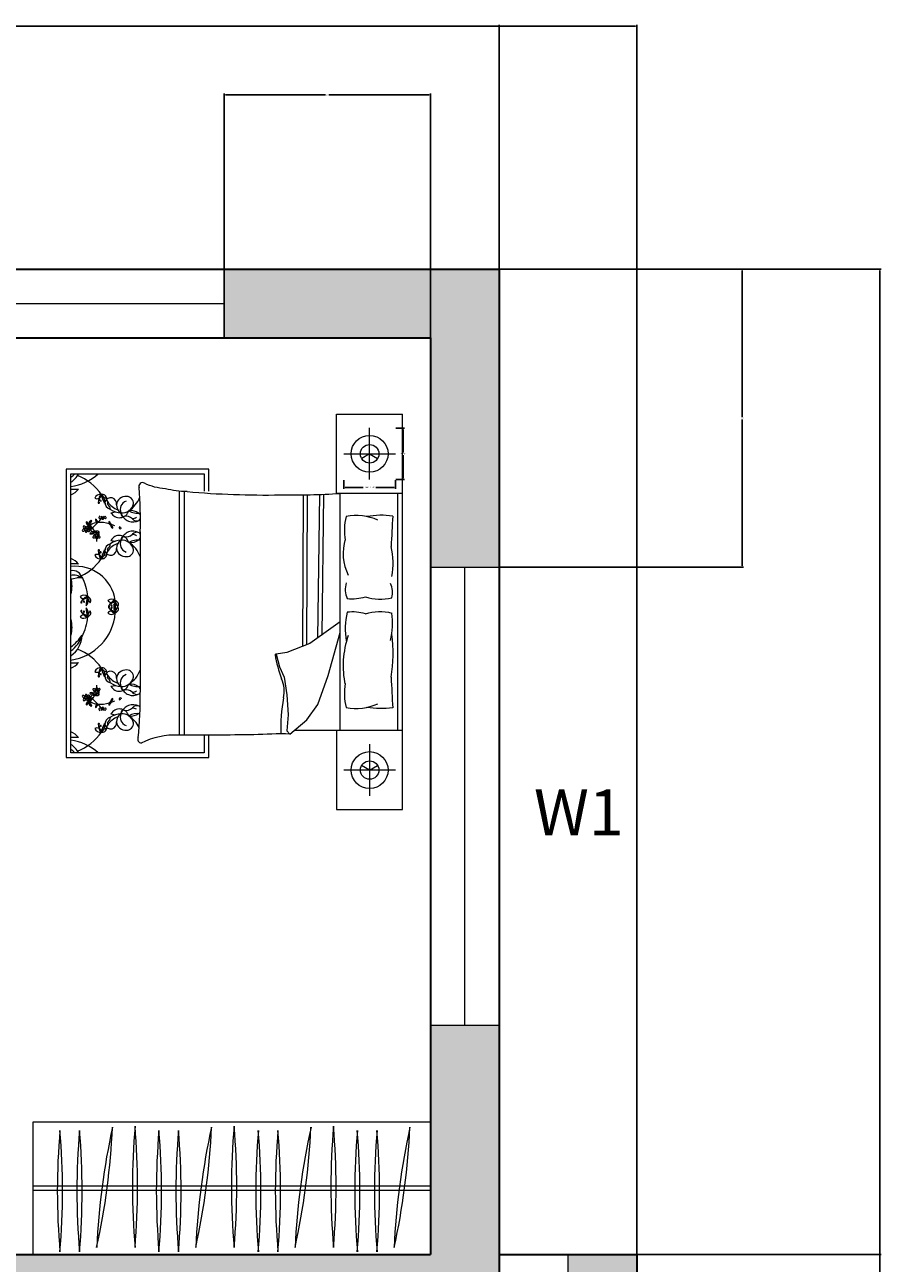
# Model space of a CAD drawing. Units: inches. Extents: x 5 to 421, y -617 to 43.
# Tile 15 of 15: x 308 to 421, y -119 to 43. Entities that reach past the tile are written whole.
import ezdxf

# ---------------------------------------------------------------- set-up
doc = ezdxf.new("R2010")
doc.units = ezdxf.units.IN
doc.header["$MEASUREMENT"] = 0
for name, color, linetype, lineweight in [('A-ANNO-DIMS', 2, 'Continuous', 18), ('A-ANNO-TEXT', 7, 'Continuous', 18), ('A-FLOR-CASE', 8, 'Continuous', 18), ('A-FURN', 8, 'Continuous', 13), ('A-GLAZ', 4, 'Continuous', 18), ('A-WALL', 7, 'Continuous', 35)]:
    doc.layers.add(name, color=color, linetype=linetype, lineweight=lineweight)
doc.layers.add('A-WALL-PATT', color=251, linetype='Continuous', lineweight=13, true_color=0x636466)
doc.styles.get("Standard").update_dxf_attribs({"font": 'arial.ttf'})
doc.dimstyles.get("Standard").update_dxf_attribs({"dimtxt": 0.18, "dimasz": 0.18, "dimexe": 0.18, "dimexo": 0.0625, "dimgap": 0.09, "dimtad": 0, "dimtih": 1, "dimtoh": 1, "dimdec": 0, "dimzin": 0, "dimdsep": 46, "dimlunit": 3, "dimtxsty": 'Standard', "dimcen": 0.09, "dimadec": 0, "dimazin": 0, "dimtfac": 1, "dimtdec": 0, "dimtofl": 0, "dimtmove": 0, "dimatfit": 3, "dimfxl": 1, "dimtolj": 1, "dimtzin": 0, "dimarcsym": 0})

# ---------------------------------------------------------------- blocks, each defined once
blk = doc.blocks.new('WINDOW-W1-60')
for p, q in [((0, 9), (60, 9)), ((0, 0), (0, 9)), ((60, 9), (60, 0)), ((0, 4.5), (60, 4.5)), ((60, 0), (0, 0))]:
    blk.add_line(p, q)
blk = doc.blocks.new('WARDROBE-52')
for p, q in [((52, 17.33), (0, 17.33)), ((0, 17.33), (0, 0)), ((52, 17.33), (52, 0)), ((52, 8.96), (0, 8.96)), ((52, 8.38), (0, 8.38)), ((52, 0), (0, 0))]:
    blk.add_line(p, q)
for centre, start, end in [((94.39, 8.32), 175.0028, 184.9972), ((-87.33, 8.32), 355.0028, 4.9972), ((96.95, 8.32), 175.0028, 184.9972), ((-84.76, 8.32), 355.0028, 4.9972), ((-80.71, 20.66), 347.508, 357.5023), ((99.46, -3.04), 167.508, 177.5023), ((104.22, 8.88), 175.0028, 184.9972), ((-77.5, 8.88), 355.0028, 4.9972), ((107.34, 8.32), 175.0028, 184.9972), ((-74.38, 8.32), 355.0028, 4.9972), ((109.91, 8.32), 175.0028, 184.9972), ((-71.81, 8.32), 355.0028, 4.9972), ((-67.75, 20.66), 347.508, 357.5023), ((112.41, -3.04), 167.508, 177.5023), ((117.17, 8.88), 175.0028, 184.9972), ((-64.54, 8.88), 355.0028, 4.9972), ((120.35, 8.32), 175.0028, 184.9972), ((-61.37, 8.32), 355.0028, 4.9972), ((122.91, 8.32), 175.0028, 184.9972), ((-58.8, 8.32), 355.0028, 4.9972), ((125.42, -3.04), 167.508, 177.5023), ((-54.75, 20.66), 347.508, 357.5023), ((130.18, 8.88), 175.0028, 184.9972), ((-51.54, 8.88), 355.0028, 4.9972), ((133.3, 8.32), 175.0028, 184.9972), ((-48.42, 8.32), 355.0028, 4.9972), ((135.87, 8.32), 175.0028, 184.9972), ((-45.85, 8.32), 355.0028, 4.9972), ((138.37, -3.04), 167.508, 177.5023), ((-41.79, 20.66), 347.508, 357.5023)]:
    blk.add_arc(centre, 91.2, start, end)
blk = doc.blocks.new('BEDSIDE-LAMP-SINGLE')
for p, q in [((3.38, 0), (3.38, 6.76)), ((0, 3.38), (6.76, 3.38))]:
    blk.add_line(p, q)
for points in [[(3.38, 3.38), (2.34, 2.78)], [(3.38, 3.38), (4.43, 2.78)]]:
    blk.add_lwpolyline(points)
for radius in [2.41, 1.21]:
    blk.add_circle((3.38, 3.38), radius)
blk = doc.blocks.new('*D50')
at = {"layer": 'A-ANNO-DIMS', "color": 0, "lineweight": -2, "transparency": 16777216}
for p, q in [((350.09, -16.74), (350.09, -17.87)), ((350.27, -17.69), (352.64, -17.69)), ((356.67, -17.69), (354.3, -17.69)), ((356.85, -16.74), (356.85, -17.87))]:
    blk.add_line(p, q, dxfattribs=at)
at = {"layer": 'A-ANNO-DIMS', "color": 0, "transparency": 16777216}
for points in [[(350.27, -17.66), (350.27, -17.72), (350.09, -17.69)], [(356.67, -17.66), (356.67, -17.72), (356.85, -17.69)]]:
    blk.add_solid(points, dxfattribs=at)
at = {"layer": 'Defpoints', "color": 0, "transparency": 16777216}
for p in [(350.09, -16.68), (356.85, -16.68), (356.85, -17.69)]:
    blk.add_point(p, dxfattribs=at)
at = {"layer": 'A-ANNO-DIMS', "color": 0, "transparency": 16777216, "insert": (353.47, -17.69), "char_height": 0.18, "attachment_point": 5}
blk.add_mtext('\\A1;LAMP 7 TYP.', dxfattribs=at)
blk = doc.blocks.new('*D51')
at = {"layer": 'A-ANNO-DIMS', "color": 0, "lineweight": -2, "transparency": 16777216}
for p, q in [((356.91, -9.92), (358.04, -9.92)), ((357.86, -10.1), (357.86, -13.12)), ((357.86, -16.5), (357.86, -13.48)), ((356.91, -16.68), (358.04, -16.68))]:
    blk.add_line(p, q, dxfattribs=at)
at = {"layer": 'A-ANNO-DIMS', "color": 0, "transparency": 16777216}
for points in [[(357.83, -10.1), (357.89, -10.1), (357.86, -9.92)], [(357.83, -16.5), (357.89, -16.5), (357.86, -16.68)]]:
    blk.add_solid(points, dxfattribs=at)
at = {"layer": 'Defpoints', "color": 0, "transparency": 16777216}
for p in [(356.85, -9.92), (357.86, -9.92), (356.85, -16.68)]:
    blk.add_point(p, dxfattribs=at)
at = {"layer": 'A-ANNO-DIMS', "color": 0, "transparency": 16777216, "insert": (357.86, -13.3), "char_height": 0.18, "attachment_point": 5}
blk.add_mtext('\\A1;7 TYP.', dxfattribs=at)
blk = doc.blocks.new('*D54')
at = {"layer": 'A-ANNO-DIMS', "color": 0, "lineweight": -2, "transparency": 16777216}
for p, q in [((37.42, 10.94), (37.42, 42.86)), ((37.6, 42.68), (212.65, 42.68)), ((388.24, 42.68), (213.19, 42.68)), ((388.42, -118.06), (388.42, 42.86))]:
    blk.add_line(p, q, dxfattribs=at)
at = {"layer": 'A-ANNO-DIMS', "color": 0, "transparency": 16777216}
for points in [[(37.6, 42.71), (37.6, 42.65), (37.42, 42.68)], [(388.24, 42.71), (388.24, 42.65), (388.42, 42.68)]]:
    blk.add_solid(points, dxfattribs=at)
at = {"layer": 'Defpoints', "color": 0, "transparency": 16777216}
for p in [(37.42, 42.68), (37.42, 10.88), (388.42, -118.12)]:
    blk.add_point(p, dxfattribs=at)
at = {"layer": 'A-ANNO-DIMS', "color": 0, "transparency": 16777216, "insert": (212.92, 42.68), "char_height": 0.18, "attachment_point": 5}
blk.add_mtext('\\A1;351', dxfattribs=at)
blk = doc.blocks.new('*D55')
at = {"layer": 'A-ANNO-DIMS', "color": 0, "lineweight": -2, "transparency": 16777216}
for p, q in [((370.48, 10.88), (420.4, 10.88)), ((420.22, 10.7), (420.22, -286.69)), ((420.22, -584.44), (420.22, -287.05)), ((169.48, -584.62), (420.4, -584.62))]:
    blk.add_line(p, q, dxfattribs=at)
at = {"layer": 'A-ANNO-DIMS', "color": 0, "transparency": 16777216}
for points in [[(420.19, 10.7), (420.25, 10.7), (420.22, 10.88)], [(420.19, -584.44), (420.25, -584.44), (420.22, -584.62)]]:
    blk.add_solid(points, dxfattribs=at)
at = {"layer": 'Defpoints', "color": 0, "transparency": 16777216}
for p in [(370.42, 10.88), (169.42, -584.62), (420.22, -584.62)]:
    blk.add_point(p, dxfattribs=at)
at = {"layer": 'A-ANNO-DIMS', "color": 0, "transparency": 16777216, "insert": (420.22, -286.87), "char_height": 0.18, "attachment_point": 5}
blk.add_mtext('\\A1;595.5', dxfattribs=at)
blk = doc.blocks.new('*D58')
at = {"layer": 'A-ANNO-DIMS', "color": 0, "lineweight": -2, "transparency": 16777216}
for p, q in [((334.42, 1.94), (334.42, 33.86)), ((334.6, 33.68), (347.7, 33.68)), ((361.24, 33.68), (348.14, 33.68)), ((361.42, 1.94), (361.42, 33.86))]:
    blk.add_line(p, q, dxfattribs=at)
at = {"layer": 'A-ANNO-DIMS', "color": 0, "transparency": 16777216}
for points in [[(334.6, 33.71), (334.6, 33.65), (334.42, 33.68)], [(361.24, 33.71), (361.24, 33.65), (361.42, 33.68)]]:
    blk.add_solid(points, dxfattribs=at)
at = {"layer": 'Defpoints', "color": 0, "transparency": 16777216}
for p in [(361.42, 33.68), (334.42, 1.88), (361.42, 1.88)]:
    blk.add_point(p, dxfattribs=at)
at = {"layer": 'A-ANNO-DIMS', "color": 0, "transparency": 16777216, "insert": (347.92, 33.68), "char_height": 0.18, "attachment_point": 5}
blk.add_mtext('\\A1;27', dxfattribs=at)
blk = doc.blocks.new('*D59')
at = {"layer": 'A-ANNO-DIMS', "color": 0, "lineweight": -2, "transparency": 16777216}
for p, q in [((370.48, 10.88), (402.4, 10.88)), ((402.22, 10.7), (402.22, -8.44)), ((402.22, -27.94), (402.22, -8.8)), ((370.48, -28.12), (402.4, -28.12))]:
    blk.add_line(p, q, dxfattribs=at)
at = {"layer": 'A-ANNO-DIMS', "color": 0, "transparency": 16777216}
for points in [[(402.19, 10.7), (402.25, 10.7), (402.22, 10.88)], [(402.19, -27.94), (402.25, -27.94), (402.22, -28.12)]]:
    blk.add_solid(points, dxfattribs=at)
at = {"layer": 'Defpoints', "color": 0, "transparency": 16777216}
for p in [(370.42, 10.88), (370.42, -28.12), (402.22, -28.12)]:
    blk.add_point(p, dxfattribs=at)
at = {"layer": 'A-ANNO-DIMS', "color": 0, "transparency": 16777216, "insert": (402.22, -8.62), "char_height": 0.18, "attachment_point": 5}
blk.add_mtext('\\A1;39', dxfattribs=at)
blk = doc.blocks.new('*D64')
at = {"layer": 'A-ANNO-DIMS', "color": 0, "lineweight": -2, "transparency": 16777216}
for p, q in [((388.48, -118.12), (420.4, -118.12)), ((420.22, -118.3), (420.22, -136.31)), ((420.22, -154.69), (420.22, -136.68)), ((388.48, -154.87), (420.4, -154.87))]:
    blk.add_line(p, q, dxfattribs=at)
at = {"layer": 'A-ANNO-DIMS', "color": 0, "transparency": 16777216}
for points in [[(420.19, -118.3), (420.25, -118.3), (420.22, -118.12)], [(420.19, -154.69), (420.25, -154.69), (420.22, -154.87)]]:
    blk.add_solid(points, dxfattribs=at)
at = {"layer": 'Defpoints', "color": 0, "transparency": 16777216}
for p in [(388.42, -118.12), (388.42, -154.87), (420.22, -154.87)]:
    blk.add_point(p, dxfattribs=at)
at = {"layer": 'A-ANNO-DIMS', "color": 0, "transparency": 16777216, "insert": (420.22, -136.49), "char_height": 0.18, "attachment_point": 5}
blk.add_mtext('\\A1;36.75', dxfattribs=at)
blk = doc.blocks.new('*D72')
at = {"layer": 'A-ANNO-DIMS', "color": 0, "lineweight": -2, "transparency": 16777216}
for p, q in [((370.42, -118.06), (370.42, 42.86)), ((370.6, 42.68), (379.21, 42.68)), ((388.24, 42.68), (379.63, 42.68)), ((388.42, -118.06), (388.42, 42.86))]:
    blk.add_line(p, q, dxfattribs=at)
at = {"layer": 'A-ANNO-DIMS', "color": 0, "transparency": 16777216}
for points in [[(370.6, 42.71), (370.6, 42.65), (370.42, 42.68)], [(388.24, 42.71), (388.24, 42.65), (388.42, 42.68)]]:
    blk.add_solid(points, dxfattribs=at)
at = {"layer": 'Defpoints', "color": 0, "transparency": 16777216}
for p in [(388.42, 42.68), (370.42, -118.12), (388.42, -118.12)]:
    blk.add_point(p, dxfattribs=at)
at = {"layer": 'A-ANNO-DIMS', "color": 0, "transparency": 16777216, "insert": (379.42, 42.68), "char_height": 0.18, "attachment_point": 5}
blk.add_mtext('\\A1;18', dxfattribs=at)

msp = doc.modelspace()

# ---------------------------------------------------------------- hatches: boundary and pattern name
at = {"layer": 'A-WALL-PATT'}
h = msp.add_hatch(color=256, dxfattribs=at)
h.dxf.hatch_style = 1
h.paths.add_polyline_path([(46.4196, -88.1188), (37.4196, -88.1188), (37.4196, -166.6119), (46.4196, -166.6119), (46.4196, -122.6188), (135.4196, -122.6188), (135.4196, -120.3688), (135.4196, -118.1188), (46.4196, -118.1188)])
h.paths.add_polyline_path([(82.4196, 10.8812), (37.4196, 10.8812), (37.4196, -28.1188), (46.4196, -28.1188), (46.4196, 1.8812), (82.4196, 1.8812)])
h.paths.add_polyline_path([(215.5968, 10.8812), (142.4196, 10.8812), (142.4196, 1.8812), (178.4196, 1.8812), (178.4196, -118.1188), (175.4196, -118.1188), (175.4196, -122.6188), (182.9196, -122.6188), (182.9196, -80.6188), (211.9196, -80.6188), (211.9196, -78.3688), (211.9196, -76.1188), (182.9196, -76.1188), (182.9196, 1.8812), (215.5968, 1.8812)])
h.paths.add_polyline_path([(274.4196, 10.8812), (239.5968, 10.8812), (239.5968, 1.8812), (242.9196, 1.8812), (242.9196, -76.1188), (239.9196, -76.1188), (239.9196, -80.6188), (242.9196, -80.6188), (242.9196, -83.6188), (247.4196, -83.6188), (247.4196, 1.8812), (274.4196, 1.8812)])
h.paths.add_polyline_path([(370.4196, 10.8812), (334.4196, 10.8812), (334.4196, 1.8812), (361.4196, 1.8812), (361.4196, -28.1188), (370.4196, -28.1188)])
h.paths.add_polyline_path([(370.4196, -88.1188), (361.4196, -88.1188), (361.4196, -118.1188), (247.4196, -118.1188), (247.4196, -115.1188), (242.9196, -115.1188), (242.9196, -118.1188), (220.4196, -118.1188), (220.4196, -158.6188), (224.9196, -158.6188), (224.9196, -122.6188), (326.9196, -122.6188), (326.9196, -170.7662), (331.4196, -170.7662), (331.4196, -122.6188), (370.4196, -122.6188)])
h.paths.add_polyline_path([(388.4196, -122.6188), (388.4196, -118.1188), (379.4196, -118.1188), (379.4196, -122.6188), (379.4196, -154.8688), (388.4196, -154.8688)])
h.paths.add_polyline_path([(388.4196, -214.8688), (379.4196, -214.8688), (379.4196, -247.1188), (388.4196, -247.1188)])
h.paths.add_polyline_path([(371.0265, -242.6188), (331.4196, -242.6188), (331.4196, -239.6188), (326.9196, -239.6188), (326.9196, -242.6188), (224.9196, -242.6188), (224.9196, -206.6188), (220.4196, -206.6188), (220.4196, -343.6188), (224.9196, -343.6188), (229.4196, -343.6188), (229.4196, -247.1188), (261.5265, -247.1188), (261.5265, -276.1188), (263.7765, -276.1188), (266.0265, -276.1188), (266.0265, -247.1188), (362.0265, -247.1188), (362.0265, -265.1188), (371.0265, -265.1188), (371.0265, -247.1188)])
h.paths.add_polyline_path([(371.0265, -289.1188), (362.0265, -289.1188), (362.0265, -307.1188), (266.0265, -307.1188), (266.0265, -304.1188), (261.5265, -304.1188), (261.5265, -307.1188), (261.5265, -311.6188), (362.0265, -311.6188), (362.0265, -353.6188), (371.0265, -353.6188)])
h.paths.add_polyline_path([(371.0265, -413.6188), (362.0265, -413.6188), (362.0265, -455.6188), (325.7231, -455.6188), (325.7231, -464.6188), (361.4196, -464.6188), (371.0265, -464.6188)])
h.paths.add_polyline_path([(265.7231, -455.6188), (229.4196, -455.6188), (229.4196, -383.6188), (220.4196, -383.6188), (220.4196, -386.6188), (207.4649, -386.6188), (207.4649, -395.6188), (220.4196, -395.6188), (220.4196, -455.6188), (216.0568, -455.6188), (216.0568, -464.6188), (265.7231, -464.6188)])
h.paths.add_polyline_path([(169.4196, -386.6188), (137.9196, -386.6188), (137.9196, -395.6188), (160.4196, -395.6188), (160.4196, -424.2032), (169.4196, -424.2032)])
h.paths.add_polyline_path([(169.4196, -453.7423), (160.4196, -453.7423), (160.4196, -464.6188), (169.4196, -464.6188)])
h.paths.add_polyline_path([(46.4196, -575.6188), (37.4196, -575.6188), (37.4196, -584.6188), (46.4196, -584.6188)])
h.paths.add_polyline_path([(169.4196, -575.6188), (160.4196, -575.6188), (160.4196, -579.5504), (160.4196, -584.6188), (169.4196, -584.6188)])
h.paths.add_polyline_path([(46.4196, -226.6119), (37.4196, -226.6119), (37.4196, -292.8008), (46.4196, -292.8008)])
h.paths.add_polyline_path([(46.4196, -352.8008), (37.4196, -352.8008), (37.4196, -395.6188), (77.9196, -395.6188), (77.9196, -386.6188), (46.4196, -386.6188)])

# ---------------------------------------------------------------- linework, layer by layer
at = {"layer": 'A-FURN'}
for p, q in [((357.7786, -59.8679), (357.7786, -8.1231)), ((313.7731, -15.314), (313.7731, -53.0381)), ((332.4131, -15.314), (313.7731, -15.314)), ((314.3727, -15.9136), (331.8135, -15.9136)), ((314.3727, -52.4385), (314.3727, -15.9136)), ((331.8135, -15.9136), (331.8135, -18.1945)), ((332.4131, -18.1836), (332.4131, -15.314)), ((328.5405, -18.1879), (328.5405, -50.1153)), ((329.1859, -18.237), (329.1859, -50.1152)), ((344.7603, -18.6551), (344.6789, -38.5095)), ((345.2915, -18.6578), (345.2134, -38.3066)), ((346.9207, -18.6311), (346.6554, -37.4202)), ((347.4517, -18.611), (347.1935, -37.0336)), ((349.6014, -49.519), (349.6014, -18.4721)), ((357.1144, -18.4721), (357.1144, -49.519)), ((319.6188, -21.0128), (320.2035, -20.8984)), ((323.4576, -23.4909), (323.4576, -44.5001)), ((319.6188, -24.6292), (320.2035, -24.7436)), ((349.6014, -35.3037), (345.6545, -38.1392)), ((348.0635, -42.3314), (349.6014, -36.6889)), ((345.6545, -38.1392), (342.617, -39.2921)), ((342.617, -39.2921), (341.2554, -39.5017)), ((341.2554, -39.5017), (341.6744, -41.1786)), ((341.6744, -41.1786), (342.3028, -42.5411)), ((319.6188, -43.723), (320.2035, -43.6086)), ((342.3028, -42.5411), (342.617, -44.8468)), ((346.7019, -46.1045), (348.0635, -42.3314)), ((342.617, -44.8468), (342.8265, -47.4669)), ((345.2355, -48.0957), (346.7019, -46.1045)), ((319.6188, -47.3394), (320.2035, -47.4538)), ((342.8265, -47.4669), (342.617, -49.563)), ((343.036, -49.9823), (345.2355, -48.0957)), ((331.8135, -50.1123), (331.8135, -52.4385)), ((332.4131, -53.0381), (332.4131, -50.1112)), ((342.617, -49.563), (343.036, -49.9823)), ((357.7786, -49.519), (343.5761, -49.519)), ((313.7731, -53.0381), (332.4131, -53.0381)), ((331.8135, -52.4385), (314.3727, -52.4385))]:
    msp.add_line(p, q, dxfattribs=at)
for points in [[(357.7786, -18.4721), (349.1545, -18.4721), (349.1545, -8.1231), (357.7786, -8.1231)], [(349.1545, -49.519), (349.1545, -59.8679), (357.7786, -59.8679)]]:
    msp.add_lwpolyline(points, dxfattribs=at)
for points in [[(329.5933, -18.2512, -0.05611182), (326.7463, -17.8758, -0.09534134), (324.0041, -17.1485)], [(356.489, -21.4442, 0.07489676), (353.1091, -21.5069, -0.47281659)], [(352.92, -32.0283, 0.14098958), (356.3681, -32.1318, 0.23524475)], [(352.92, -34.238, -0.14098958), (356.3681, -34.1345, -0.23524475)], [(356.489, -46.5469, -0.07489676), (353.1091, -46.4842, 0.47281659)], [(338.2979, -50.0905, -0.00124232), (328.4799, -50.1153, 0.12720156), (323.5869, -51.1526)]]:
    msp.add_lwpolyline(points, format="xyb", dxfattribs=at)
for centre in [(316.3547, -23.1403), (317.7438, -24.0023), (316.3547, -45.2119), (317.7438, -44.3499)]:
    msp.add_circle(centre, 0.1318, dxfattribs=at)
for centre, radius, start, end in [((312.5573, -14.2729), 3.2926, 303.461725, 330.111571), ((311.9434, -13.0882), 4.1032, 306.303565, 316.481422), ((313.4621, -10.8831), 6.7571, 277.744957, 311.885603), ((312.794, -22.4435), 6.7571, 34.386545, 68.590793), ((323.7415, -17.5403), 0.4716, 56.173584, 203.478142), ((273.1309, -21.9063), 50.3517, 358.196492, 4.759758), ((313.3189, -16.117), 2.7474, 292.554743, 318.95456), ((314.7955, -8.5912), 9.3489, 267.408107, 273.651905), ((318.2109, -19.3594), 0.7493, 77.711531, 159.038678), ((317.8063, -18.6104), 0.5643, 238.463314, 358.286895), ((319.6569, -19.752), 1.7089, 138.840165, 177.935195), ((318.6272, -19.1167), 0.5528, 117.682699, 223.776193), ((318.3087, -19.4405), 0.044, 223.772923, 159.733291), ((318.5033, -19.1714), 0.5602, 2.951587, 103.727964), ((322.9851, -17.6027), 4.7271, 192.517257, 207.18239), ((317.746, -19.4941), 1.0683, 345.465349, 54.234293), ((319.3556, -18.0262), 1.1541, 211.382672, 255.296877), ((319.5768, -19.8293), 0.7766, 350.263976, 160.868843), ((318.7353, -19.6694), 0.476, 333.975548, 53.268054), ((321.5692, -20.1137), 1.2365, 84.944852, 172.885747), ((321.6942, -19.7555), 0.8736, 354.485571, 91.05378), ((319.8137, -17.4741), 3.9163, 303.667122, 336.354674), ((339.8971, 102.5942), 121.2839, 265.126493, 270.885464), ((343.2775, 74.2895), 92.9769, 269.071824, 273.900032), ((318.033, -19.6934), 0.0839, 177.935195, 11.483395), ((318.0753, -19.6848), 0.0408, 11.483395, 127.940894), ((319.8105, -19.6429), 0.9698, 175.969018, 254.304497), ((318.5213, -20.6875), 1.0328, 6.166203, 51.582546), ((321.2862, -18.2896), 2.4429, 211.261374, 251.704505), ((321.0893, -18.2667), 2.7768, 236.288284, 266.507596), ((320.7339, -20.3714), 1.2864, 209.908541, 343.133701), ((321.844, -19.8987), 1.5031, 182.359103, 234.040141), ((322.038, -20.5997), 1.2008, 111.581867, 201.422148), ((321.0478, -19.4872), 1.5563, 265.293344, 346.920995), ((322.144, -22.7228), 1.9956, 122.70113, 126.34448), ((323.0748, -18.9105), 2.1438, 238.821784, 280.751011), ((322.144, -22.7228), 1.9956, 55.785047, 94.730373), ((322.8852, -21.5658), 0.6232, 17.418575, 52.324972), ((316.5469, -22.2903), 0.1471, 124.353798, 214.392331), ((316.763, -22.3121), 0.3431, 190.305679, 287.195801), ((316.8616, -22.1899), 0.3983, 176.970073, 248.291288), ((319.7043, -20.0903), 3.8498, 212.678403, 216.37461), ((316.7272, -22.2831), 0.1523, 216.37461, 291.754782), ((318.075, -24.4211), 2.1485, 124.003336, 132.491708), ((315.8653, -24.6924), 2.2952, 63.781945, 68.291288), ((317.0908, -22.9263), 0.3651, 128.320824, 208.816232), ((317.0909, -22.3895), 0.3431, 122.815476, 187.399174), ((316.8263, -22.5314), 0.115, 289.360543, 111.754782), ((316.9126, -22.5319), 0.115, 221.870337, 44.264579), ((317.4332, -22.8658), 0.6007, 157.230483, 229.063527), ((317.2415, -22.4338), 0.3983, 109.479868, 177.68284), ((317.2312, -22.6675), 0.3535, 174.454356, 220.618813), ((315.2213, -24.6421), 2.5772, 30.544017, 49.817977), ((317.0282, -22.1815), 0.1471, 56.863595, 146.902126), ((317.104, -22.3453), 0.1523, 148.884407, 224.264579), ((320.2695, -24.2561), 3.8498, 145.188198, 148.884407), ((318.075, -24.4211), 2.1485, 94.756021, 119.204084), ((322.6498, -27.5142), 7.0702, 132.241244, 142.174439), ((319.0806, -21.8873), 1.4593, 178.326386, 187.130238), ((317.5048, -22.0898), 0.2717, 11.325614, 64.46214), ((318.4267, -21.699), 0.8178, 190.258782, 210.655993), ((317.8783, -22.0324), 0.2483, 188.343222, 274.286854), ((318.0962, -21.8949), 0.4337, 210.655993, 242.634143), ((318.4244, -21.5222), 0.8314, 218.210121, 226.307119), ((317.8097, -22.2207), 0.1054, 325.765747, 67.441651), ((314.5365, -18.6958), 4.9131, 313.154125, 322.045905), ((318.1829, -26.5562), 4.2857, 73.584179, 93.827683), ((318.1495, -21.6474), 0.1011, 142.473712, 265.053037), ((318.2829, -21.6271), 0.2176, 127.762086, 169.040263), ((318.1672, -21.443), 0.3062, 265.053037, 338.361764), ((318.5727, -21.862), 0.4001, 113.427571, 137.610371), ((318.5269, -21.4476), 0.1318, 183.276835, 356.723165), ((318.6238, -21.686), 0.2156, 139.788918, 227.679152), ((318.555, -21.7615), 0.1136, 227.679152, 350.348696), ((318.1153, -21.6832), 0.4314, 353.085162, 15.717093), ((318.3984, -21.7349), 0.2724, 350.348696, 43.653825), ((318.9032, -21.4534), 0.3169, 198.726271, 262.503155), ((318.6516, -21.6012), 0.1259, 1.108054, 91.867469), ((318.8878, -21.6691), 0.1018, 255.235561, 54.924803), ((318.731, -21.6298), 0.2198, 11.563728, 52.635797), ((320.8217, -22.1955), 1.4593, 178.326386, 187.130238), ((319.2459, -22.3981), 0.2717, 11.325614, 64.46214), ((320.1678, -22.0073), 0.8178, 190.258782, 210.655993), ((319.6194, -22.3406), 0.2483, 188.343222, 274.286854), ((319.8373, -22.2032), 0.4337, 210.655993, 242.634143), ((320.1655, -21.8305), 0.8314, 218.210121, 226.307119), ((319.5508, -22.529), 0.1054, 325.765747, 67.441651), ((319.8475, -22.7216), 0.2483, 147.533168, 233.476805), ((320.0716, -22.5944), 0.4337, 179.185879, 211.164033), ((319.6491, -22.6931), 0.1054, 354.378377, 96.054275), ((318.1829, -26.5562), 4.2857, 63.003195, 69.894078), ((321.2746, -21.1859), 0.3212, 167.304058, 285.147127), ((322.5178, -20.5708), 1.649, 199.282177, 299.1751), ((321.6357, -22.5199), 1.0608, 41.565306, 105.147127), ((322.2194, -20.3219), 1.4874, 277.435988, 299.914865), ((323.0088, -21.3024), 0.7743, 221.565306, 293.835407), ((322.8852, -21.5658), 0.6232, 314.451692, 343.365665), ((357.0945, -23.29), 6.9345, 165.103933, 191.036887), ((351.7522, -28.0365), 6.6691, 65.1316, 101.758341), ((848.9287, -49.9656), 493.265, 176.685209, 177.149775), ((315.9773, -23.3401), 0.1011, 142.473712, 265.053037), ((316.1107, -23.3198), 0.2176, 61.219585, 169.040263), ((315.995, -23.1357), 0.3062, 265.053037, 338.361764), ((316.2542, -22.872), 0.2601, 157.408573, 261.438586), ((316.1074, -22.8634), 0.1306, 58.049899, 135.626809), ((316.4005, -23.5547), 0.4001, 113.427571, 137.610371), ((316.2436, -22.9452), 0.0873, 172.906013, 277.131983), ((315.9566, -23.1051), 0.4155, 14.755814, 58.049899), ((316.4516, -23.3787), 0.2156, 139.788918, 227.679152), ((316.3829, -23.4542), 0.1136, 227.679152, 350.348696), ((316.538, -22.9948), 0.1797, 36.104556, 181.428111), ((315.9431, -23.3759), 0.4314, 353.085162, 15.717093), ((316.2263, -23.4276), 0.2724, 350.348696, 43.653825), ((316.7311, -23.1461), 0.3169, 198.726271, 262.503155), ((316.4334, -22.8534), 0.1814, 270.064508, 331.150746), ((316.588, -22.8965), 0.2073, 221.84125, 265.787705), ((316.4794, -23.2939), 0.1259, 1.108054, 91.867469), ((316.5868, -22.9748), 0.1291, 263.752558, 41.70535), ((316.5589, -23.3225), 0.2198, 11.563728, 86.365034), ((316.7157, -23.3618), 0.1018, 255.235561, 54.924803), ((317.1573, -22.8993), 0.4364, 207.704258, 254.35163), ((316.8732, -23.1495), 0.6007, 270.278003, 342.111048), ((317.2737, -23.9001), 0.4249, 98.722715, 159.337457), ((317.0606, -23.3546), 0.4364, 244.989901, 291.637274), ((316.6403, -23.1743), 0.4249, 340.004072, 40.618813), ((317.1556, -23.1307), 0.3535, 278.722715, 324.887172), ((317.0935, -23.4184), 0.3651, 290.5253, 358.5375), ((317.3663, -24.202), 0.1011, 142.473712, 265.053037), ((317.4998, -24.1818), 0.2176, 61.219585, 169.040263), ((317.384, -23.9976), 0.3062, 265.053037, 338.361764), ((317.6432, -23.7339), 0.2601, 157.408573, 261.438586), ((317.4964, -23.7253), 0.1306, 58.049899, 135.626809), ((317.8055, -23.3142), 0.3651, 182.849877, 266.122608), ((317.6636, -23.0563), 0.3535, 231.760733, 277.925193), ((317.9396, -22.9935), 0.6007, 214.536861, 286.369906), ((317.7896, -24.4166), 0.4001, 113.427571, 137.610371), ((317.6326, -23.8071), 0.0873, 172.906013, 277.131983), ((317.3457, -23.9671), 0.4155, 14.755814, 58.049899), ((315.2213, -24.6421), 2.5772, 23.050074, 23.847739), ((317.8406, -24.2407), 0.2156, 139.788918, 227.679152), ((317.7709, -23.8273), 0.4249, 37.310451, 97.925193), ((317.9271, -23.8568), 0.1797, 36.104556, 181.428111), ((317.3322, -24.2378), 0.4314, 353.085162, 15.717093), ((317.8188, -23.2437), 0.4364, 265.010636, 311.65801), ((317.6153, -24.2895), 0.2724, 350.348696, 43.653825), ((318.1201, -24.008), 0.3169, 198.726271, 262.503155), ((317.8224, -23.7153), 0.1814, 270.064508, 331.150746), ((317.977, -23.7584), 0.2073, 221.84125, 265.787705), ((317.8685, -24.1558), 0.1259, 1.108054, 91.867469), ((317.9759, -23.8368), 0.1291, 263.752558, 41.70535), ((317.9479, -24.1845), 0.2198, 11.563728, 86.365034), ((318.1047, -24.2237), 0.1018, 255.235561, 54.924803), ((320.7339, -25.2706), 1.2864, 16.866299, 150.091459), ((320.5432, -21.7303), 1.4593, 234.689789, 243.493639), ((320.4003, -22.3956), 0.8178, 211.164033, 231.561245), ((320.5551, -22.4811), 0.8314, 195.512908, 203.609906), ((319.6205, -23.0237), 0.2717, 357.357882, 50.494412), ((320.7875, -22.9695), 0.0997, 12.70507, 190.438449), ((320.8489, -22.9582), 0.1622, 190.438449, 10.413559), ((321.2746, -24.456), 0.3212, 74.852873, 192.695942), ((322.5178, -25.0712), 1.649, 60.8249, 160.717823), ((321.6357, -23.1221), 1.0608, 254.852873, 318.434694), ((322.2194, -25.3201), 1.4874, 60.085135, 82.564012), ((323.0088, -24.3396), 0.7743, 66.164593, 138.434694), ((322.8852, -24.0762), 0.6232, 23.285643, 45.548308), ((317.7719, -24.3161), 0.1136, 227.679152, 350.348696), ((315.2213, -24.6421), 2.5772, 357.107093, 4.758526), ((318.033, -25.9486), 0.0839, 348.516605, 182.064805), ((317.746, -26.1479), 1.0683, 305.765707, 14.534651), ((322.9851, -28.0393), 4.7271, 152.81761, 167.482743), ((319.8105, -25.9991), 0.9698, 105.695503, 184.030982), ((319.5768, -25.8127), 0.7766, 199.131157, 9.736024), ((318.7353, -25.9726), 0.476, 306.731946, 26.024452), ((318.5213, -24.9545), 1.0328, 308.417454, 353.833797), ((321.2862, -27.3524), 2.4429, 108.295495, 148.738626), ((321.0893, -27.3753), 2.7768, 93.492404, 123.711716), ((321.844, -25.7433), 1.5031, 125.959859, 177.640897), ((321.5692, -25.5283), 1.2365, 187.114253, 275.055148), ((322.038, -25.0423), 1.2008, 158.577852, 248.418133), ((321.0478, -26.1547), 1.5563, 13.079005, 94.706656), ((322.144, -22.9192), 1.9956, 233.65552, 237.29887), ((321.6942, -25.8865), 0.8736, 268.94622, 5.514429), ((323.0748, -26.7315), 2.1438, 79.713345, 121.178216), ((322.144, -22.9192), 1.9956, 265.269627, 304.214953), ((319.8137, -28.1679), 3.9163, 21.494132, 56.332878), ((322.8852, -24.0762), 0.6232, 307.675028, 336.714357), ((356.5836, -26.2828), 6.5869, 163.825361, 206.123892), ((347.4347, -27.5856), 9.0964, 348.8159, 13.657286), ((313.3189, -29.525), 2.7474, 41.04544, 67.445257), ((312.794, -23.1985), 6.7571, 291.409207, 325.613455), ((317.8063, -27.0316), 0.5643, 1.713105, 121.536686), ((318.2109, -26.2826), 0.7493, 200.961322, 282.288469), ((319.6569, -25.89), 1.7089, 182.064805, 221.159835), ((318.0753, -25.9572), 0.0408, 232.059106, 348.516605), ((318.6272, -26.5253), 0.5528, 136.223807, 242.317301), ((318.2808, -26.1934), 0.0731, 200.281654, 136.223807), ((318.5033, -26.4706), 0.5602, 256.272036, 357.048413), ((319.3556, -27.6158), 1.1541, 104.703123, 148.617328), ((314.7955, -37.0508), 9.3489, 86.348095, 92.591893), ((315.0224, -33.2524), 5.2296, 8.180341, 97.136446), ((314.6582, -29.8011), 1.2129, 10.926149, 103.610181), ((314.8247, -30.7126), 1.5337, 48.095132, 107.139124), ((310.8199, -30.627), 3.7156, 343.543107, 17.020201), ((315.5003, -32.5763), 3.0253, 83.380464, 111.882968), ((309.8429, -32.5167), 6.7571, 4.462329, 27.414598), ((353.0158, -31.0756), 2.7431, 161.459272, 204.98174), ((353.9087, -31.4218), 2.5598, 343.897443, 26.656258), ((308.905, -32.099), 5.4943, 4.378724, 5.635738), ((305.1407, -34.9928), 9.8185, 19.721715, 19.902844), ((316.0761, -32.546), 0.7493, 47.787318, 129.114465), ((316.0991, -31.695), 0.5643, 208.539099, 328.362682), ((317.1336, -33.6076), 1.7089, 108.915948, 148.010978), ((316.5579, -32.5433), 0.5528, 87.758486, 193.85198), ((321.0901, -33.4051), 4.7271, 162.593037, 177.258174), ((315.606, -32.4308), 1.0683, 315.541131, 24.310082), ((317.7333, -31.9616), 1.1541, 181.458456, 225.372663), ((316.4233, -32.5289), 0.5602, 333.027371, 73.803749), ((319.6953, -33.0633), 0.7493, 47.787318, 129.114465), ((351.1906, -25.9286), 6.3402, 264.012888, 285.829277), ((315.7553, -32.7468), 0.0839, 148.010978, 341.559179), ((315.7553, -33.8806), 0.0839, 18.440821, 211.989022), ((317.1336, -33.0197), 1.7089, 211.989022, 251.084052), ((315.7963, -32.7604), 0.0408, 341.559179, 98.016679), ((315.7963, -33.8669), 0.0408, 261.983321, 18.440821), ((316.5579, -34.084), 0.5528, 166.14802, 272.241514), ((316.0922, -33.9692), 0.0731, 230.075459, 166.14802), ((316.1204, -32.6651), 0.044, 193.979118, 129.809076), ((321.0901, -33.2222), 4.7271, 182.741826, 197.406963), ((315.606, -34.1966), 1.0683, 335.689918, 44.458869), ((317.7333, -34.6657), 1.1541, 134.627337, 178.541544), ((316.4233, -34.0984), 0.5602, 286.196251, 26.972629), ((319.7183, -32.2123), 0.5643, 208.539099, 328.362682), ((319.7183, -34.415), 0.5643, 31.637318, 151.460901), ((319.3746, -33.2641), 0.0839, 148.010978, 341.559179), ((319.3746, -33.3632), 0.0839, 18.440821, 211.989022), ((320.7528, -34.125), 1.7089, 108.915948, 148.010978), ((320.7528, -32.5024), 1.7089, 211.989022, 251.084052), ((319.4155, -33.2778), 0.0408, 341.559179, 98.016679), ((319.4155, -33.3496), 0.0408, 261.983321, 18.440821), ((320.1772, -33.0607), 0.5528, 87.758486, 193.85198), ((320.1772, -33.5667), 0.5528, 166.14802, 272.241514), ((319.7114, -33.4518), 0.0731, 230.075459, 166.14802), ((319.7397, -33.1825), 0.044, 193.979118, 129.809076), ((319.2252, -32.9481), 1.0683, 315.541131, 24.310082), ((324.7094, -33.9225), 4.7271, 162.593037, 177.258174), ((319.2252, -33.6792), 1.0683, 335.689918, 44.458869), ((324.7094, -32.7049), 4.7271, 182.741826, 197.406963), ((320.0425, -33.0463), 0.5602, 333.027371, 73.803749), ((321.3525, -32.479), 1.1541, 181.458456, 225.372663), ((320.0425, -33.5811), 0.5602, 286.196251, 26.972629), ((321.3525, -34.1484), 1.1541, 134.627337, 178.541544), ((359.3976, -36.1815), 9.125, 166.376244, 190.138311), ((351.1906, -40.3377), 6.3402, 74.170723, 95.987112), ((313.4621, -33.5933), 6.7571, 277.744957, 355.537671), ((310.8199, -36.0004), 3.7156, 342.979799, 16.456893), ((308.905, -34.5283), 5.4943, 354.364262, 355.621276), ((305.1407, -31.6345), 9.8185, 340.097156, 340.278285), ((316.0991, -34.9324), 0.5643, 31.637318, 151.460901), ((316.0761, -34.0814), 0.7493, 230.885535, 312.212682), ((309.8429, -34.1106), 6.7571, 332.585402, 355.537671), ((319.6953, -33.564), 0.7493, 230.885535, 312.212682), ((347.2485, -35.4933), 9.2203, 346.040041, 8.475073), ((312.5573, -36.9831), 3.2926, 303.461725, 358.728033), ((310.7898, -33.6421), 6.1034, 305.946958, 325.987662), ((311.9434, -35.7984), 4.1032, 306.303565, 342.149621), ((362.0236, -41.0507), 12.0272, 160.738476, 191.960255), ((337.7646, -39.4568), 18.7665, 350.503017, 7.780417), ((312.794, -45.1537), 6.7571, 34.386545, 68.590793), ((341.2132, -39.6192), 0.1249, 70.246365, 181.137655), ((360.8091, -35.9091), 20.0671, 190.66171, 199.880578), ((314.7955, -31.3014), 9.3489, 267.408107, 273.651905), ((313.3189, -38.8272), 2.7474, 292.554743, 318.95456), ((318.2109, -42.0696), 0.7493, 77.711531, 159.038678), ((317.8063, -41.3205), 0.5643, 238.463314, 358.286895), ((319.6569, -42.4622), 1.7089, 138.840165, 177.935195), ((318.6272, -41.8269), 0.5528, 117.682699, 223.776193), ((318.3087, -42.1507), 0.044, 223.772923, 159.733291), ((318.5033, -41.8816), 0.5602, 2.951587, 103.727964), ((319.3556, -40.7364), 1.1541, 211.382672, 255.296877), ((317.746, -42.2042), 1.0683, 345.465349, 54.234293), ((322.9851, -40.3129), 4.7271, 192.517257, 207.18239), ((319.5768, -42.5394), 0.7766, 350.263976, 160.868843), ((318.7353, -42.3796), 0.476, 333.975548, 53.268054), ((321.5692, -42.8239), 1.2365, 84.944852, 172.885747), ((321.6942, -42.4657), 0.8736, 354.485571, 91.05378), ((319.8137, -40.1843), 3.9163, 303.667122, 338.505868), ((315.2213, -43.7101), 2.5772, 355.241474, 2.892907), ((318.033, -42.4036), 0.0839, 177.935195, 11.483395), ((318.0753, -42.395), 0.0408, 11.483395, 127.940894), ((319.8105, -42.3531), 0.9698, 175.969018, 254.304497), ((318.5213, -43.3976), 1.0328, 6.166203, 51.582546), ((321.2862, -40.9997), 2.4429, 211.261374, 251.704505), ((321.0893, -40.9768), 2.7768, 236.288284, 266.507596), ((320.7339, -43.0816), 1.2864, 209.908541, 343.133701), ((321.844, -42.6089), 1.5031, 182.359103, 234.040141), ((322.038, -43.3099), 1.2008, 111.581867, 201.422148), ((321.0478, -42.1974), 1.5563, 265.293344, 346.920995), ((322.144, -45.4329), 1.9956, 122.70113, 126.34448), ((323.0748, -41.6206), 2.1438, 238.821784, 280.286655), ((322.144, -45.4329), 1.9956, 55.785047, 94.730373), ((338.0821, -44.4288), 4.2121, 348.660801, 23.738416), ((357.0945, -44.7011), 6.9345, 168.963113, 194.896067), ((848.9287, -18.0255), 493.265, 182.850225, 183.314791), ((315.9773, -45.0121), 0.1011, 94.946963, 217.526288), ((316.1107, -45.0323), 0.2176, 190.959737, 298.780415), ((315.995, -45.2165), 0.3062, 21.638236, 94.946963), ((316.2542, -45.4802), 0.2601, 98.561414, 202.591427), ((316.4005, -44.7975), 0.4001, 222.389629, 246.572429), ((316.2436, -45.407), 0.0873, 82.868017, 187.093987), ((315.9566, -45.247), 0.4155, 301.950101, 345.244186), ((316.4516, -44.9734), 0.2156, 132.320848, 220.211082), ((316.3829, -44.898), 0.1136, 9.651304, 132.320848), ((316.538, -45.3573), 0.1797, 178.571889, 323.895444), ((315.9431, -44.9763), 0.4314, 344.282907, 6.914838), ((316.2263, -44.9246), 0.2724, 316.346175, 9.651304), ((316.7311, -45.2061), 0.3169, 97.496845, 161.273729), ((316.588, -45.4557), 0.2073, 94.212295, 138.15875), ((316.4334, -45.4988), 0.1814, 28.849254, 89.935492), ((316.4794, -45.0583), 0.1259, 268.132531, 358.891946), ((316.5589, -45.0296), 0.2198, 273.634966, 348.436272), ((316.5868, -45.3773), 0.1291, 318.29465, 96.247442), ((316.7157, -44.9904), 0.1018, 305.075197, 104.764439), ((317.0908, -45.4259), 0.3651, 151.183768, 231.679176), ((317.1573, -45.4528), 0.4364, 105.64837, 152.295742), ((317.4332, -45.4863), 0.6007, 130.936473, 202.769517), ((317.0606, -44.9975), 0.4364, 68.362726, 115.010099), ((316.8732, -45.2027), 0.6007, 17.888952, 89.721997), ((317.2737, -44.4521), 0.4249, 200.662543, 261.277285), ((315.2213, -43.7101), 2.5772, 310.182023, 329.455983), ((316.6403, -45.1779), 0.4249, 319.381187, 19.995928), ((322.6498, -40.8379), 7.0702, 217.825561, 227.758756), ((317.1556, -45.2215), 0.3535, 35.112828, 81.277285), ((317.0935, -44.9338), 0.3651, 1.4625, 69.4747), ((317.3663, -44.1502), 0.1011, 94.946963, 217.526288), ((317.4998, -44.1704), 0.2176, 190.959737, 298.780415), ((317.384, -44.3545), 0.3062, 21.638236, 94.946963), ((317.6432, -44.6182), 0.2601, 98.561414, 202.591427), ((317.4964, -44.6268), 0.1306, 224.373191, 301.950101), ((317.8055, -45.0379), 0.3651, 93.877392, 177.150123), ((317.9396, -45.3587), 0.6007, 73.630094, 145.463139), ((317.6636, -45.2958), 0.3535, 82.074807, 128.239267), ((317.7896, -43.9355), 0.4001, 222.389629, 246.572429), ((317.6326, -44.5451), 0.0873, 82.868017, 187.093987), ((317.3457, -44.3851), 0.4155, 301.950101, 345.244186), ((315.2213, -43.7101), 2.5772, 336.152261, 336.949926), ((317.8406, -44.1115), 0.2156, 132.320848, 220.211082), ((317.7719, -44.036), 0.1136, 9.651304, 132.320848), ((317.7709, -44.5248), 0.4249, 262.074807, 322.689549), ((317.3322, -44.1144), 0.4314, 344.282907, 6.914838), ((317.9271, -44.4954), 0.1797, 178.571889, 323.895444), ((317.8188, -45.1085), 0.4364, 48.34199, 94.989364), ((317.6153, -44.0627), 0.2724, 316.346175, 9.651304), ((318.1201, -44.3441), 0.3169, 97.496845, 161.273729), ((317.977, -44.5937), 0.2073, 94.212295, 138.15875), ((317.8224, -44.6369), 0.1814, 28.849254, 89.935492), ((317.8685, -44.1963), 0.1259, 268.132531, 358.891946), ((317.9479, -44.1677), 0.2198, 273.634966, 348.436272), ((317.9759, -44.5154), 0.1291, 318.29465, 96.247442), ((318.1047, -44.1284), 0.1018, 305.075197, 104.764439), ((320.5432, -46.6218), 1.4593, 116.506361, 125.310211), ((320.4003, -45.9565), 0.8178, 128.438755, 148.835967), ((319.6205, -45.3285), 0.2717, 309.505588, 2.642118), ((320.7875, -45.3827), 0.0997, 169.561551, 347.29493), ((320.8489, -45.394), 0.1622, 349.586441, 169.561551), ((321.2746, -43.8961), 0.3212, 167.304058, 285.147127), ((322.5178, -43.281), 1.649, 199.282177, 299.1751), ((321.6357, -45.2301), 1.0608, 41.565306, 105.147127), ((322.2194, -43.0321), 1.4874, 277.435988, 299.914865), ((323.0088, -44.0126), 0.7743, 221.565306, 293.835407), ((269.5943, -45.1176), 53.8669, 354.311309, 0.656746), ((322.8852, -44.2759), 0.6232, 23.285643, 52.324972), ((322.8852, -44.2759), 0.6232, 314.451692, 336.770992), ((361.36, -49.0967), 19.5292, 168.660801, 182.54812), ((316.1074, -45.4888), 0.1306, 224.373191, 301.950101), ((316.5469, -46.0618), 0.1471, 145.607669, 235.646202), ((316.763, -46.0401), 0.3431, 72.804199, 169.694321), ((316.8616, -46.1622), 0.3983, 111.708712, 183.029927), ((319.7043, -48.2619), 3.8498, 143.62539, 147.321597), ((316.7272, -46.0691), 0.1523, 68.245218, 143.62539), ((318.075, -43.9311), 2.1485, 227.508292, 235.996664), ((315.8653, -43.6598), 2.2952, 291.708712, 296.218055), ((317.0909, -45.9627), 0.3431, 172.600826, 237.184524), ((316.8263, -45.8208), 0.115, 248.245218, 70.639457), ((316.9126, -45.8203), 0.115, 315.735421, 138.129663), ((317.2415, -45.9184), 0.3983, 182.31716, 250.520132), ((317.2312, -45.6846), 0.3535, 139.381187, 185.545644), ((317.0282, -46.1707), 0.1471, 213.097874, 303.136405), ((317.104, -46.0068), 0.1523, 135.735421, 211.115593), ((320.2695, -44.0961), 3.8498, 211.115593, 214.811802), ((318.075, -43.9311), 2.1485, 240.795916, 265.243979), ((319.0806, -46.4649), 1.4593, 172.869762, 181.673614), ((318.4267, -46.6532), 0.8178, 149.344007, 169.741218), ((317.5048, -46.2624), 0.2717, 295.53786, 348.674386), ((317.8783, -46.3198), 0.2483, 85.713146, 171.656778), ((318.0962, -46.4573), 0.4337, 117.365857, 149.344007), ((318.4244, -46.83), 0.8314, 133.692881, 141.789879), ((317.8097, -46.1315), 0.1054, 292.558349, 34.234253), ((318.1829, -41.796), 4.2857, 266.172317, 286.415821), ((314.5365, -49.6563), 4.9131, 37.954095, 46.845875), ((318.1495, -46.7048), 0.1011, 94.946963, 217.526288), ((318.2829, -46.725), 0.2176, 190.959737, 232.237914), ((318.1672, -46.9092), 0.3062, 21.638236, 94.946963), ((318.5727, -46.4902), 0.4001, 222.389629, 246.572429), ((318.5269, -46.9045), 0.1318, 3.276835, 176.723165), ((318.6238, -46.6661), 0.2156, 132.320848, 220.211082), ((318.555, -46.5907), 0.1136, 9.651304, 132.320848), ((318.1153, -46.669), 0.4314, 344.282907, 6.914838), ((318.3984, -46.6173), 0.2724, 316.346175, 9.651304), ((318.9032, -46.8988), 0.3169, 97.496845, 161.273729), ((318.6516, -46.751), 0.1259, 268.132531, 358.891946), ((318.8878, -46.6831), 0.1018, 305.075197, 104.764439), ((318.731, -46.7223), 0.2198, 307.364203, 348.436272), ((320.8217, -46.1566), 1.4593, 172.869762, 181.673614), ((320.1678, -46.3449), 0.8178, 149.344007, 169.741218), ((319.2459, -45.9541), 0.2717, 295.53786, 348.674386), ((319.6194, -46.0115), 0.2483, 85.713146, 171.656778), ((319.8373, -46.149), 0.4337, 117.365857, 149.344007), ((320.1655, -46.5217), 0.8314, 133.692881, 141.789879), ((319.5508, -45.8232), 0.1054, 292.558349, 34.234253), ((319.8475, -45.6306), 0.2483, 126.523195, 212.466832), ((320.7339, -47.9808), 1.2864, 16.866299, 150.091459), ((320.0716, -45.7577), 0.4337, 148.835967, 180.814121), ((319.6491, -45.659), 0.1054, 263.945725, 5.621623), ((318.1829, -41.796), 4.2857, 290.105922, 296.996805), ((320.5551, -45.8711), 0.8314, 156.390094, 164.487092), ((321.2746, -47.1662), 0.3212, 74.852873, 192.695942), ((322.5178, -47.7813), 1.649, 60.8249, 160.717823), ((321.6357, -45.8322), 1.0608, 254.852873, 318.434694), ((322.2194, -48.0303), 1.4874, 60.085135, 82.564012), ((323.0088, -47.0498), 0.7743, 66.164593, 138.434694), ((322.8852, -46.7864), 0.6232, 26.441992, 45.548308), ((351.7522, -39.9545), 6.6691, 258.241659, 294.8684), ((318.033, -48.6587), 0.0839, 348.516605, 182.064805), ((322.9851, -50.7494), 4.7271, 152.81761, 167.482743), ((317.746, -48.8581), 1.0683, 305.765707, 14.534651), ((319.8105, -48.7092), 0.9698, 105.695503, 184.030982), ((319.5768, -48.5229), 0.7766, 199.131157, 9.736024), ((318.7353, -48.6828), 0.476, 306.731946, 26.024452), ((318.5213, -47.6647), 1.0328, 308.417454, 353.833797), ((321.2862, -50.0626), 2.4429, 108.295495, 148.738626), ((321.0893, -50.0855), 2.7768, 93.492404, 123.711716), ((321.844, -48.4535), 1.5031, 125.959859, 177.640897), ((321.5692, -48.2384), 1.2365, 187.114253, 275.055148), ((322.038, -47.7524), 1.2008, 158.577852, 248.418133), ((321.0478, -48.8649), 1.5563, 13.079005, 94.706656), ((322.144, -45.6294), 1.9956, 233.65552, 237.29887), ((321.6942, -48.5967), 0.8736, 268.94622, 5.514429), ((323.0748, -49.4417), 2.1438, 80.844576, 121.178216), ((322.144, -45.6294), 1.9956, 265.269627, 304.214953), ((319.8137, -50.8781), 3.9163, 26.700344, 56.332878), ((322.8852, -46.7864), 0.6232, 307.675028, 329.970699), ((313.3189, -52.2352), 2.7474, 41.04544, 67.445257), ((312.794, -45.9087), 6.7571, 291.409207, 325.613455), ((317.8063, -49.7418), 0.5643, 1.713105, 121.536686), ((318.2109, -48.9928), 0.7493, 200.961322, 282.288469), ((319.6569, -48.6002), 1.7089, 182.064805, 221.159835), ((318.0753, -48.6673), 0.0408, 232.059106, 348.516605), ((318.6272, -49.2354), 0.5528, 136.223807, 242.317301), ((318.2808, -48.9036), 0.0731, 200.281654, 136.223807), ((319.3556, -50.3259), 1.1541, 104.703123, 148.617328), ((318.5033, -49.1808), 0.5602, 256.272036, 357.048413), ((341.7496, -97.4269), 47.4621, 88.446955, 94.170589), ((314.7955, -59.761), 9.3489, 86.348095, 92.591893), ((313.4621, -57.4691), 6.7571, 48.114397, 82.255043), ((312.5573, -54.0793), 3.2926, 29.888429, 56.538275), ((323.62, -50.6763), 0.4775, 152.658759, 266.020019), ((311.9434, -55.2639), 4.1032, 43.518578, 53.696435)]:
    msp.add_arc(centre, radius, start, end, dxfattribs=at)
at = {"layer": 'A-GLAZ'}
msp.add_line((379.4196, -122.6188), (379.4196, -118.1188), dxfattribs=at)
at = {"layer": 'A-WALL'}
for p, q in [((37.4196, 10.8812), (370.4196, 10.8812)), ((370.4196, 10.8812), (370.4196, -122.6188)), ((247.4196, 1.8812), (361.4196, 1.8812)), ((361.4196, 1.8812), (361.4196, -118.1188)), ((247.4196, -118.1188), (361.4196, -118.1188)), ((370.4196, -118.1188), (388.4196, -118.1188)), ((388.4196, -118.1188), (388.4196, -122.6188))]:
    msp.add_line(p, q, dxfattribs=at)

# ---------------------------------------------------------------- block references
at = {"layer": 'A-FLOR-CASE'}
msp.add_blockref('WARDROBE-52', (309.4187, -118.1188), dxfattribs=at)
at = {"layer": 'A-FURN'}
msp.add_blockref('BEDSIDE-LAMP-SINGLE', (350.0859, -16.6783), dxfattribs=at)
at = {"layer": 'A-FURN', "rotation": 180}
msp.add_blockref('BEDSIDE-LAMP-SINGLE', (356.8472, -51.3128), dxfattribs=at)
at = {"layer": 'A-GLAZ'}
msp.add_blockref('WINDOW-W1-60', (274.4196, 1.8812), dxfattribs=at)
at = {"layer": 'A-GLAZ', "rotation": 90.00000000000011}
msp.add_blockref('WINDOW-W1-60', (370.4196, -88.1188), dxfattribs=at)

# ---------------------------------------------------------------- texts
at = {"layer": 'A-ANNO-TEXT', "insert": (374.9674, -57.2341), "char_height": 6, "attachment_point": 1}
msp.add_mtext('W1', dxfattribs=at)

# ---------------------------------------------------------------- dimensions: what is measured, and where the dimension line sits
at = {"layer": 'A-ANNO-DIMS'}
for base, p1, p2, picture, middle in [((37.4196, 42.6812), (388.4196, -118.1188), (37.4196, 10.8812), '*D54', (212.9196, 42.6812)), ((388.4196, 42.6812), (370.4196, -118.1188), (388.4196, -118.1188), '*D72', (379.4196, 42.6812)), ((361.4196, 33.6812), (334.4196, 1.8812), (361.4196, 1.8812), '*D58', (347.9196, 33.6812))]:
    dim = msp.add_linear_dim(base=base, p1=p1, p2=p2, dimstyle='Standard', override={"dimdec": 0, "dimlfac": 1, "dimrnd": 0, "dimzin": 0, "dimdsep": 46, "dimlunit": 2}, dxfattribs=at)
    dim.commit()
    dim.dimension.update_dxf_attribs({"geometry": picture, "text_midpoint": middle})
for base, p1, p2, angle, override, picture, middle in [((420.2196, -584.6188), (370.4196, 10.8812), (169.4196, -584.6188), 90, {"dimdec": 1, "dimlfac": 1, "dimrnd": 0, "dimzin": 0, "dimdsep": 46, "dimlunit": 2}, '*D55', (420.2196, -286.8688)), ((402.2196, -28.1188), (370.4196, 10.8812), (370.4196, -28.1188), 270, {"dimdec": 0, "dimlfac": 1, "dimrnd": 0, "dimzin": 0, "dimdsep": 46, "dimlunit": 2}, '*D59', (402.2196, -8.6188)), ((420.2196, -154.8688), (388.4196, -118.1188), (388.4196, -154.8688), 90, {"dimdec": 2, "dimlfac": 1, "dimrnd": 0, "dimzin": 0, "dimdsep": 46, "dimlunit": 2}, '*D64', (420.2196, -136.4938))]:
    dim = msp.add_linear_dim(base=base, p1=p1, p2=p2, angle=angle, dimstyle='Standard', override=override, dxfattribs=at)
    dim.commit()
    dim.dimension.update_dxf_attribs({"geometry": picture, "text_midpoint": middle})
dim = msp.add_linear_dim(base=(357.8614, -9.917), p1=(356.8472, -16.6783), p2=(356.8472, -9.917), angle=90, text='<> TYP.', dimstyle='Standard', override={"dimdec": 0, "dimlfac": 1, "dimrnd": 0, "dimzin": 0, "dimdsep": 46, "dimlunit": 2}, dxfattribs=at)
dim.commit()
dim.dimension.update_dxf_attribs({"geometry": '*D51', "text_midpoint": (357.8614, -13.2976)})
dim = msp.add_linear_dim(base=(356.8472, -17.6925), p1=(350.0859, -16.6783), p2=(356.8472, -16.6783), text='LAMP <> TYP.', dimstyle='Standard', override={"dimdec": 0, "dimlfac": 1, "dimrnd": 0, "dimzin": 0, "dimdsep": 46, "dimlunit": 2}, dxfattribs=at)
dim.commit()
dim.dimension.update_dxf_attribs({"geometry": '*D50', "text_midpoint": (353.4665, -17.6925)})

doc.saveas('drawing.dxf')
